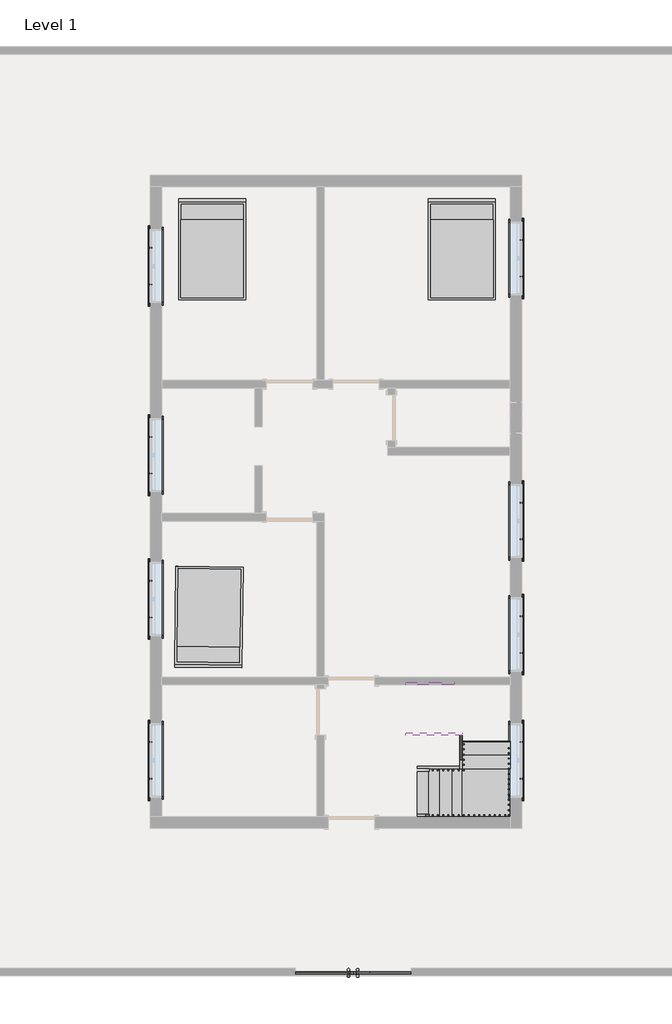
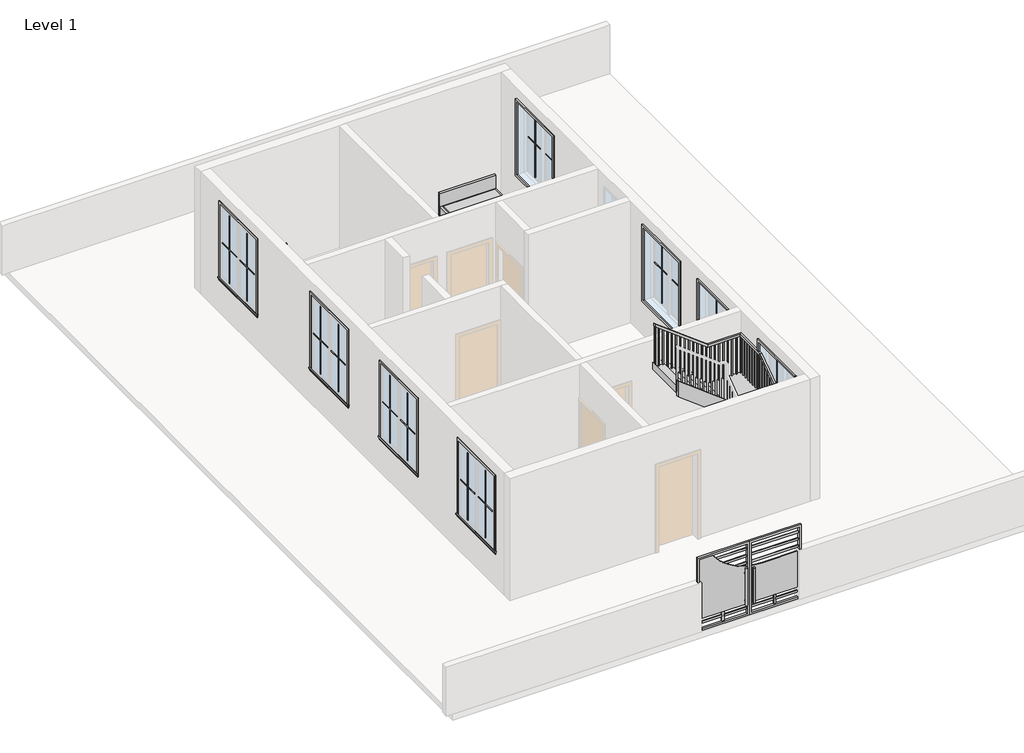
# One storey, part 2 of 2: 33 proxies, 5 members, 3 furniture elements, 1 railing, 1 stair flight.
"""IFC4 building model written with IfcOpenShell, lengths in millimetres."""

from ifc_helpers import new_model, si_unit, frame, origin, place, context, project, spatial, polyline, outline, extrude, faceted_brep, transform, mapped, element, save
from components import generic_models_113f6068, muntin_pattern_2x2_muntin_pattern_2x2_bff912c5, muntin_pattern_2x2_muntin_pattern_2x2_c2194282, trim_window_exterior_flat_with_sill_e04b3088, trim_window_interior_flat_picture_frame_2a7685fe, bed_17739_bed_17739_15c61121, stair_flight_3d22c4e0

model = new_model("IFC4")

# Units and contexts
model_context = context("Model", 3, world=origin())
ifc_project = project(units=[si_unit("LENGTHUNIT", "METRE", prefix="MILLI")], contexts=[model_context])

# Site, building, storey
site = spatial("IfcSite", under=ifc_project)
building = spatial("IfcBuilding", under=site)
storey = spatial("IfcBuildingStorey", under=building, Name="Level 1", Elevation=0.0)

# Proxies
placement = place(None, origin())
generic_models_shape = generic_models_113f6068(model_context)
element("IfcBuildingElementProxy", 1, Name="Generic Models", at=placement, inside=storey, context=model_context, shape_type="MappedRepresentation", body=[
    mapped(generic_models_shape, transform((-917.7018997, -9199.4071712, 0.0), x_axis=(1.0, 0.0, 0.0), y_axis=(0.0, 1.0, 0.0), z_axis=(0.0, 0.0, 1.0))),
])
muntin_pattern_2x2_muntin_pattern_2x2_shape = muntin_pattern_2x2_muntin_pattern_2x2_bff912c5(model_context)
element("IfcBuildingElementProxy", 2, Name="Muntin Pattern_2x2 : Muntin Pattern_2x2", ObjectType="Muntin Pattern_2x2 : Muntin Pattern_2x2", at=placement, inside=storey, context=model_context, shape_type="MappedRepresentation", body=[
    mapped(muntin_pattern_2x2_muntin_pattern_2x2_shape, transform((-4903.510885, -5396.5975571, 984.25), x_axis=(0.0, 1.0, 0.0), y_axis=(-1.0, 0.0, 0.0), z_axis=(0.0, 0.0, 1.0))),
])
element("IfcBuildingElementProxy", 3, Name="Muntin Pattern_2x2 : Muntin Pattern_2x2", ObjectType="Muntin Pattern_2x2 : Muntin Pattern_2x2", at=placement, inside=storey, context=model_context, shape_type="MappedRepresentation", body=[
    mapped(muntin_pattern_2x2_muntin_pattern_2x2_shape, transform((2392.639115, -4675.8725571, 984.25), x_axis=(0.0, -1.0, 0.0), y_axis=(1.0, 0.0, 0.0), z_axis=(0.0, 0.0, 1.0))),
])
element("IfcBuildingElementProxy", 4, Name="Muntin Pattern_2x2 : Muntin Pattern_2x2", ObjectType="Muntin Pattern_2x2 : Muntin Pattern_2x2", at=placement, inside=storey, context=model_context, shape_type="MappedRepresentation", body=[
    mapped(muntin_pattern_2x2_muntin_pattern_2x2_shape, transform((2392.639115, -2199.3725571, 984.25), x_axis=(0.0, -1.0, 0.0), y_axis=(1.0, 0.0, 0.0), z_axis=(0.0, 0.0, 1.0))),
])
element("IfcBuildingElementProxy", 5, Name="Muntin Pattern_2x2 : Muntin Pattern_2x2", ObjectType="Muntin Pattern_2x2 : Muntin Pattern_2x2", at=placement, inside=storey, context=model_context, shape_type="MappedRepresentation", body=[
    mapped(muntin_pattern_2x2_muntin_pattern_2x2_shape, transform((2392.639115, 35.8274429, 984.25), x_axis=(0.0, -1.0, 0.0), y_axis=(1.0, 0.0, 0.0), z_axis=(0.0, 0.0, 1.0))),
])
element("IfcBuildingElementProxy", 6, Name="Muntin Pattern_2x2 : Muntin Pattern_2x2", ObjectType="Muntin Pattern_2x2 : Muntin Pattern_2x2", at=placement, inside=storey, context=model_context, shape_type="MappedRepresentation", body=[
    mapped(muntin_pattern_2x2_muntin_pattern_2x2_shape, transform((-4903.510885, -2221.5975571, 984.25), x_axis=(0.0, 1.0, 0.0), y_axis=(-1.0, 0.0, 0.0), z_axis=(0.0, 0.0, 1.0))),
])
element("IfcBuildingElementProxy", 7, Name="Muntin Pattern_2x2 : Muntin Pattern_2x2", ObjectType="Muntin Pattern_2x2 : Muntin Pattern_2x2", at=placement, inside=storey, context=model_context, shape_type="MappedRepresentation", body=[
    mapped(muntin_pattern_2x2_muntin_pattern_2x2_shape, transform((-4903.510885, 610.5024429, 984.25), x_axis=(0.0, 1.0, 0.0), y_axis=(-1.0, 0.0, 0.0), z_axis=(0.0, 0.0, 1.0))),
])
element("IfcBuildingElementProxy", 8, Name="Muntin Pattern_2x2 : Muntin Pattern_2x2", ObjectType="Muntin Pattern_2x2 : Muntin Pattern_2x2", at=placement, inside=storey, context=model_context, shape_type="MappedRepresentation", body=[
    mapped(muntin_pattern_2x2_muntin_pattern_2x2_shape, transform((-4903.510885, 4331.6024429, 984.25), x_axis=(0.0, 1.0, 0.0), y_axis=(-1.0, 0.0, 0.0), z_axis=(0.0, 0.0, 1.0))),
])
element("IfcBuildingElementProxy", 9, Name="Muntin Pattern_2x2 : Muntin Pattern_2x2", ObjectType="Muntin Pattern_2x2 : Muntin Pattern_2x2", at=placement, inside=storey, context=model_context, shape_type="MappedRepresentation", body=[
    mapped(muntin_pattern_2x2_muntin_pattern_2x2_shape, transform((2392.639115, 5204.7274429, 984.25), x_axis=(0.0, -1.0, 0.0), y_axis=(1.0, 0.0, 0.0), z_axis=(0.0, 0.0, 1.0))),
])
muntin_pattern_2x2_muntin_pattern_2x2_2_shape = muntin_pattern_2x2_muntin_pattern_2x2_c2194282(model_context)
element("IfcBuildingElementProxy", 10, Name="Muntin Pattern_2x2 : Muntin Pattern_2x2", ObjectType="Muntin Pattern_2x2 : Muntin Pattern_2x2", at=placement, inside=storey, context=model_context, shape_type="MappedRepresentation", body=[
    mapped(muntin_pattern_2x2_muntin_pattern_2x2_2_shape, transform((-4903.510885, -4675.8725571, 984.25), x_axis=(0.0, -1.0, 0.0), y_axis=(1.0, 0.0, 0.0), z_axis=(0.0, 0.0, 1.0))),
])
element("IfcBuildingElementProxy", 11, Name="Muntin Pattern_2x2 : Muntin Pattern_2x2", ObjectType="Muntin Pattern_2x2 : Muntin Pattern_2x2", at=placement, inside=storey, context=model_context, shape_type="MappedRepresentation", body=[
    mapped(muntin_pattern_2x2_muntin_pattern_2x2_2_shape, transform((2392.639115, -5396.5975571, 984.25), x_axis=(0.0, 1.0, 0.0), y_axis=(-1.0, 0.0, 0.0), z_axis=(0.0, 0.0, 1.0))),
])
element("IfcBuildingElementProxy", 12, Name="Muntin Pattern_2x2 : Muntin Pattern_2x2", ObjectType="Muntin Pattern_2x2 : Muntin Pattern_2x2", at=placement, inside=storey, context=model_context, shape_type="MappedRepresentation", body=[
    mapped(muntin_pattern_2x2_muntin_pattern_2x2_2_shape, transform((2392.639115, -2920.0975571, 984.25), x_axis=(0.0, 1.0, 0.0), y_axis=(-1.0, 0.0, 0.0), z_axis=(0.0, 0.0, 1.0))),
])
element("IfcBuildingElementProxy", 13, Name="Muntin Pattern_2x2 : Muntin Pattern_2x2", ObjectType="Muntin Pattern_2x2 : Muntin Pattern_2x2", at=placement, inside=storey, context=model_context, shape_type="MappedRepresentation", body=[
    mapped(muntin_pattern_2x2_muntin_pattern_2x2_2_shape, transform((2392.639115, -684.8975571, 984.25), x_axis=(0.0, 1.0, 0.0), y_axis=(-1.0, 0.0, 0.0), z_axis=(0.0, 0.0, 1.0))),
])
element("IfcBuildingElementProxy", 14, Name="Muntin Pattern_2x2 : Muntin Pattern_2x2", ObjectType="Muntin Pattern_2x2 : Muntin Pattern_2x2", at=placement, inside=storey, context=model_context, shape_type="MappedRepresentation", body=[
    mapped(muntin_pattern_2x2_muntin_pattern_2x2_2_shape, transform((-4903.510885, -1500.8725571, 984.25), x_axis=(0.0, -1.0, 0.0), y_axis=(1.0, 0.0, 0.0), z_axis=(0.0, 0.0, 1.0))),
])
element("IfcBuildingElementProxy", 15, Name="Muntin Pattern_2x2 : Muntin Pattern_2x2", ObjectType="Muntin Pattern_2x2 : Muntin Pattern_2x2", at=placement, inside=storey, context=model_context, shape_type="MappedRepresentation", body=[
    mapped(muntin_pattern_2x2_muntin_pattern_2x2_2_shape, transform((-4903.510885, 1331.2274429, 984.25), x_axis=(0.0, -1.0, 0.0), y_axis=(1.0, 0.0, 0.0), z_axis=(0.0, 0.0, 1.0))),
])
element("IfcBuildingElementProxy", 16, Name="Muntin Pattern_2x2 : Muntin Pattern_2x2", ObjectType="Muntin Pattern_2x2 : Muntin Pattern_2x2", at=placement, inside=storey, context=model_context, shape_type="MappedRepresentation", body=[
    mapped(muntin_pattern_2x2_muntin_pattern_2x2_2_shape, transform((-4903.510885, 5052.3274429, 984.25), x_axis=(0.0, -1.0, 0.0), y_axis=(1.0, 0.0, 0.0), z_axis=(0.0, 0.0, 1.0))),
])
element("IfcBuildingElementProxy", 17, Name="Muntin Pattern_2x2 : Muntin Pattern_2x2", ObjectType="Muntin Pattern_2x2 : Muntin Pattern_2x2", at=placement, inside=storey, context=model_context, shape_type="MappedRepresentation", body=[
    mapped(muntin_pattern_2x2_muntin_pattern_2x2_2_shape, transform((2392.639115, 4484.0024429, 984.25), x_axis=(0.0, 1.0, 0.0), y_axis=(-1.0, 0.0, 0.0), z_axis=(0.0, 0.0, 1.0))),
])
trim_window_exterior_flat_with_sill_shape = trim_window_exterior_flat_with_sill_e04b3088(model_context)
element("IfcBuildingElementProxy", 18, Name="Trim-Window-Exterior-Flat : with Sill", ObjectType="Trim-Window-Exterior-Flat : with Sill", at=placement, inside=storey, context=model_context, shape_type="MappedRepresentation", body=[
    mapped(trim_window_exterior_flat_with_sill_shape, transform((-4913.035885, -5036.2350571, 2743.2), x_axis=(0.0, -1.0, 0.0), y_axis=(0.0, 0.0, 1.0), z_axis=(-1.0, 0.0, 0.0))),
])
element("IfcBuildingElementProxy", 19, Name="Trim-Window-Exterior-Flat : with Sill", ObjectType="Trim-Window-Exterior-Flat : with Sill", at=placement, inside=storey, context=model_context, shape_type="MappedRepresentation", body=[
    mapped(trim_window_exterior_flat_with_sill_shape, transform((2402.164115, -5036.2350571, 2743.2), x_axis=(0.0, 1.0, 0.0), y_axis=(0.0, 0.0, 1.0), z_axis=(1.0, 0.0, 0.0))),
])
element("IfcBuildingElementProxy", 20, Name="Trim-Window-Exterior-Flat : with Sill", ObjectType="Trim-Window-Exterior-Flat : with Sill", at=placement, inside=storey, context=model_context, shape_type="MappedRepresentation", body=[
    mapped(trim_window_exterior_flat_with_sill_shape, transform((2402.164115, -2559.7350571, 2743.2), x_axis=(0.0, 1.0, 0.0), y_axis=(0.0, 0.0, 1.0), z_axis=(1.0, 0.0, 0.0))),
])
element("IfcBuildingElementProxy", 21, Name="Trim-Window-Exterior-Flat : with Sill", ObjectType="Trim-Window-Exterior-Flat : with Sill", at=placement, inside=storey, context=model_context, shape_type="MappedRepresentation", body=[
    mapped(trim_window_exterior_flat_with_sill_shape, transform((2402.164115, -324.5350571, 2743.2), x_axis=(0.0, 1.0, 0.0), y_axis=(0.0, 0.0, 1.0), z_axis=(1.0, 0.0, 0.0))),
])
element("IfcBuildingElementProxy", 22, Name="Trim-Window-Exterior-Flat : with Sill", ObjectType="Trim-Window-Exterior-Flat : with Sill", at=placement, inside=storey, context=model_context, shape_type="MappedRepresentation", body=[
    mapped(trim_window_exterior_flat_with_sill_shape, transform((-4913.035885, -1861.2350571, 2743.2), x_axis=(0.0, -1.0, 0.0), y_axis=(0.0, 0.0, 1.0), z_axis=(-1.0, 0.0, 0.0))),
])
element("IfcBuildingElementProxy", 23, Name="Trim-Window-Exterior-Flat : with Sill", ObjectType="Trim-Window-Exterior-Flat : with Sill", at=placement, inside=storey, context=model_context, shape_type="MappedRepresentation", body=[
    mapped(trim_window_exterior_flat_with_sill_shape, transform((-4913.035885, 970.8649429, 2743.2), x_axis=(0.0, -1.0, 0.0), y_axis=(0.0, 0.0, 1.0), z_axis=(-1.0, 0.0, 0.0))),
])
element("IfcBuildingElementProxy", 24, Name="Trim-Window-Exterior-Flat : with Sill", ObjectType="Trim-Window-Exterior-Flat : with Sill", at=placement, inside=storey, context=model_context, shape_type="MappedRepresentation", body=[
    mapped(trim_window_exterior_flat_with_sill_shape, transform((-4913.035885, 4691.9649429, 2743.2), x_axis=(0.0, -1.0, 0.0), y_axis=(0.0, 0.0, 1.0), z_axis=(-1.0, 0.0, 0.0))),
])
element("IfcBuildingElementProxy", 25, Name="Trim-Window-Exterior-Flat : with Sill", ObjectType="Trim-Window-Exterior-Flat : with Sill", at=placement, inside=storey, context=model_context, shape_type="MappedRepresentation", body=[
    mapped(trim_window_exterior_flat_with_sill_shape, transform((2402.164115, 4844.3649429, 2743.2), x_axis=(0.0, 1.0, 0.0), y_axis=(0.0, 0.0, 1.0), z_axis=(1.0, 0.0, 0.0))),
])
trim_window_interior_flat_picture_frame_shape = trim_window_interior_flat_picture_frame_2a7685fe(model_context)
element("IfcBuildingElementProxy", 26, Name="Trim-Window-Interior-Flat : Picture Frame", ObjectType="Trim-Window-Interior-Flat : Picture Frame", at=placement, inside=storey, context=model_context, shape_type="MappedRepresentation", body=[
    mapped(trim_window_interior_flat_picture_frame_shape, transform((-4684.435885, -5036.2350571, 2743.2), x_axis=(0.0, 1.0, 0.0), y_axis=(0.0, 0.0, 1.0), z_axis=(1.0, 0.0, 0.0))),
])
element("IfcBuildingElementProxy", 27, Name="Trim-Window-Interior-Flat : Picture Frame", ObjectType="Trim-Window-Interior-Flat : Picture Frame", at=placement, inside=storey, context=model_context, shape_type="MappedRepresentation", body=[
    mapped(trim_window_interior_flat_picture_frame_shape, transform((2173.564115, -5036.2350571, 2743.2), x_axis=(0.0, -1.0, 0.0), y_axis=(0.0, 0.0, 1.0), z_axis=(-1.0, 0.0, 0.0))),
])
element("IfcBuildingElementProxy", 28, Name="Trim-Window-Interior-Flat : Picture Frame", ObjectType="Trim-Window-Interior-Flat : Picture Frame", at=placement, inside=storey, context=model_context, shape_type="MappedRepresentation", body=[
    mapped(trim_window_interior_flat_picture_frame_shape, transform((2173.564115, -2559.7350571, 2743.2), x_axis=(0.0, -1.0, 0.0), y_axis=(0.0, 0.0, 1.0), z_axis=(-1.0, 0.0, 0.0))),
])
element("IfcBuildingElementProxy", 29, Name="Trim-Window-Interior-Flat : Picture Frame", ObjectType="Trim-Window-Interior-Flat : Picture Frame", at=placement, inside=storey, context=model_context, shape_type="MappedRepresentation", body=[
    mapped(trim_window_interior_flat_picture_frame_shape, transform((2173.564115, -324.5350571, 2743.2), x_axis=(0.0, -1.0, 0.0), y_axis=(0.0, 0.0, 1.0), z_axis=(-1.0, 0.0, 0.0))),
])
element("IfcBuildingElementProxy", 30, Name="Trim-Window-Interior-Flat : Picture Frame", ObjectType="Trim-Window-Interior-Flat : Picture Frame", at=placement, inside=storey, context=model_context, shape_type="MappedRepresentation", body=[
    mapped(trim_window_interior_flat_picture_frame_shape, transform((-4684.435885, -1861.2350571, 2743.2), x_axis=(0.0, 1.0, 0.0), y_axis=(0.0, 0.0, 1.0), z_axis=(1.0, 0.0, 0.0))),
])
element("IfcBuildingElementProxy", 31, Name="Trim-Window-Interior-Flat : Picture Frame", ObjectType="Trim-Window-Interior-Flat : Picture Frame", at=placement, inside=storey, context=model_context, shape_type="MappedRepresentation", body=[
    mapped(trim_window_interior_flat_picture_frame_shape, transform((-4684.435885, 970.8649429, 2743.2), x_axis=(0.0, 1.0, 0.0), y_axis=(0.0, 0.0, 1.0), z_axis=(1.0, 0.0, 0.0))),
])
element("IfcBuildingElementProxy", 32, Name="Trim-Window-Interior-Flat : Picture Frame", ObjectType="Trim-Window-Interior-Flat : Picture Frame", at=placement, inside=storey, context=model_context, shape_type="MappedRepresentation", body=[
    mapped(trim_window_interior_flat_picture_frame_shape, transform((-4684.435885, 4691.9649429, 2743.2), x_axis=(0.0, 1.0, 0.0), y_axis=(0.0, 0.0, 1.0), z_axis=(1.0, 0.0, 0.0))),
])
element("IfcBuildingElementProxy", 33, Name="Trim-Window-Interior-Flat : Picture Frame", ObjectType="Trim-Window-Interior-Flat : Picture Frame", at=placement, inside=storey, context=model_context, shape_type="MappedRepresentation", body=[
    mapped(trim_window_interior_flat_picture_frame_shape, transform((2173.564115, 4844.3649429, 2743.2), x_axis=(0.0, -1.0, 0.0), y_axis=(0.0, 0.0, 1.0), z_axis=(-1.0, 0.0, 0.0))),
])

# Furniture
bed_17739_bed_17739_shape = bed_17739_bed_17739_15c61121(model_context)
element("IfcFurniture", 34, ObjectType="Bed_17739 : Bed_17739", at=placement, inside=storey, context=model_context, shape_type="MappedRepresentation", body=[
    mapped(bed_17739_bed_17739_shape, transform((-3693.835885, 4996.7649429, 0.0), x_axis=(1.0, 0.0, 0.0), y_axis=(0.0, 1.0, 0.0), z_axis=(0.0, 0.0, 1.0))),
])
element("IfcFurniture", 35, ObjectType="Bed_17739 : Bed_17739", at=placement, inside=storey, context=model_context, shape_type="MappedRepresentation", body=[
    mapped(bed_17739_bed_17739_shape, transform((1221.064115, 4996.7649429, 0.0), x_axis=(1.0, 0.0, 0.0), y_axis=(0.0, 1.0, 0.0), z_axis=(0.0, 0.0, 1.0))),
])
element("IfcFurniture", 36, ObjectType="Bed_17739 : Bed_17739", at=placement, inside=storey, context=model_context, shape_type="MappedRepresentation", body=[
    mapped(bed_17739_bed_17739_shape, transform((-3756.0321663, -2189.364606, 0.0), x_axis=(-0.9999334593473937, 0.011535895177843815, 0.0), y_axis=(-0.011535895177843815, -0.9999334593473937, 0.0), z_axis=(0.0, 0.0, 1.0))),
])

# Members
element("IfcMember", 37, ObjectType="Stringer - 2\" Width", at=placement, inside=storey, context=model_context, shape_type="SweptSolid", body=[
    extrude(outline(polyline([(222.6959685, 344.764115), (0.0, 344.764115), (0.0, 555.1685253), (482.9196844, 1182.964115), (867.4651993, 1182.964115), (222.6959685, 344.764115)])), frame((0.0, -5201.3350571, 0.0), z_axis=(0.0, 1.0, 0.0), x_axis=(0.0, 0.0, 1.0)), (0.0, 0.0, 1.0), 50.8),
])
element("IfcMember", 38, ObjectType="Stringer - 2\" Width", at=placement, inside=storey, context=model_context, shape_type="SweptSolid", body=[
    extrude(outline(polyline([(-5201.3350571, 695.152716), (-5201.3350571, 1069.7225362), (-4540.9350571, 1541.4368219), (-4540.9350571, 1166.8670017), (-5201.3350571, 695.152716)])), frame((1182.964115, 0.0, 0.0), z_axis=(1.0, 0.0, 0.0), x_axis=(0.0, 1.0, 0.0)), (0.0, 0.0, 1.0), 50.8),
])
element("IfcMember", 39, ObjectType="Stringer - 2\" Width", at=placement, inside=storey, context=model_context, shape_type="SweptSolid", body=[
    extrude(outline(polyline([(1369.1786616, 1233.764115), (1752.3668, 1233.764115), (2603.8715619, 116.164115), (2220.6834236, 116.164115), (1369.1786616, 1233.764115)])), frame((0.0, -4540.9350571, 0.0), z_axis=(0.0, 1.0, 0.0), x_axis=(0.0, 0.0, 1.0)), (0.0, 0.0, 1.0), 50.8),
])
element("IfcMember", 40, ObjectType="Stringer - 2\" Width", at=placement, inside=storey, context=model_context, shape_type="SweptSolid", body=[
    extrude(outline(polyline([(222.6959685, 344.764115), (0.0, 344.764115), (0.0, 555.1685253), (398.4368219, 1073.1363938), (398.4368219, 573.2272245), (222.6959685, 344.764115)])), frame((0.0, -6191.9350571, 0.0), z_axis=(0.0, 1.0, 0.0), x_axis=(0.0, 0.0, 1.0)), (0.0, 0.0, 1.0), 50.8),
])
element("IfcMember", 41, ObjectType="Stringer - 2\" Width", at=placement, inside=storey, context=model_context, shape_type="SweptSolid", body=[
    extrude(outline(polyline([(1874.4384303, 1073.5451003), (2603.8715619, 116.164115), (2220.6834236, 116.164115), (1874.4384303, 570.6106687), (1874.4384303, 1073.5451003)])), frame((0.0, -3550.3350571, 0.0), z_axis=(0.0, 1.0, 0.0), x_axis=(0.0, 0.0, 1.0)), (0.0, 0.0, 1.0), 50.8),
])

# Railing
element("IfcRailing", 42, ObjectType="Handrail - Rectangular", at=placement, inside=storey, context=model_context, shape_type="SolidModel", body=[
    faceted_brep([(344.764115, -6090.3350571, 1083.7333333), (344.764115, -6090.3350571, 1019.8686436), (344.764115, -6141.1350571, 1019.8686436), (344.764115, -6141.1350571, 1083.7333333), (1373.464115, -6090.3350571, 1867.5047619), (1390.6115203, -6090.3350571, 1816.7047619), (1390.6115203, -6141.1350571, 1816.7047619), (1373.464115, -6141.1350571, 1867.5047619), (2122.764115, -6090.3350571, 1867.5047619), (2122.764115, -6090.3350571, 1816.7047619), (2173.564115, -6141.1350571, 1816.7047619), (2173.564115, -6141.1350571, 1867.5047619), (2122.764115, -5289.3883904, 1867.5047619), (2122.764115, -5273.1087657, 1816.7047619), (2173.564115, -5273.1087657, 1816.7047619), (2173.564115, -5289.3883904, 1867.5047619), (2122.764115, -4399.3108146, 2503.2744589), (2122.764115, -4383.0311899, 2452.4744589), (2173.564115, -4383.0311899, 2452.4744589), (2173.564115, -4399.3108146, 2503.2744589), (2122.764115, -3601.1350571, 2503.2744589), (2122.764115, -3601.1350571, 2452.4744589), (2173.564115, -3550.3350571, 2452.4744589), (2173.564115, -3550.3350571, 2503.2744589), (1371.6498293, -3601.1350571, 2503.2744589), (1354.5800477, -3601.1350571, 2452.4744589), (1354.5800477, -3550.3350571, 2452.4744589), (1371.6498293, -3550.3350571, 2503.2744589), (116.164115, -3601.1350571, 3454.4), (116.164115, -3550.3350571, 3454.4), (116.164115, -3550.3350571, 3390.6683472), (116.164115, -3601.1350571, 3390.6683472)], [[[0, 1, 2, 3]], [[1, 0, 4, 5]], [[2, 1, 5, 6]], [[3, 2, 6, 7]], [[0, 3, 7, 4]], [[5, 4, 8, 9]], [[6, 5, 9, 10]], [[7, 6, 10, 11]], [[4, 7, 11, 8]], [[9, 8, 12, 13]], [[10, 9, 13, 14]], [[11, 10, 14, 15]], [[8, 11, 15, 12]], [[13, 12, 16, 17]], [[14, 13, 17, 18]], [[15, 14, 18, 19]], [[12, 15, 19, 16]], [[17, 16, 20, 21]], [[18, 17, 21, 22]], [[19, 18, 22, 23]], [[16, 19, 23, 20]], [[21, 20, 24, 25]], [[22, 21, 25, 26]], [[23, 22, 26, 27]], [[20, 23, 27, 24]], [[28, 29, 30, 31]], [[25, 24, 28, 31]], [[26, 25, 31, 30]], [[27, 26, 30, 29]], [[24, 27, 29, 28]]]),
    extrude(outline(polyline([(3306.4827412, 227.289115), (3320.9145594, 208.239115), (2370.6666667, 208.239115), (2370.6666667, 227.289115), (3306.4827412, 227.289115)])), frame((0.0, -3585.2600571, 0.0), z_axis=(0.0, 1.0, 0.0), x_axis=(0.0, 0.0, 1.0)), (0.0, 0.0, 1.0), 19.05),
    extrude(outline(polyline([(3229.5130442, 328.889115), (3243.9448624, 309.839115), (2370.6666667, 309.839115), (2370.6666667, 328.889115), (3229.5130442, 328.889115)])), frame((0.0, -3585.2600571, 0.0), z_axis=(0.0, 1.0, 0.0), x_axis=(0.0, 0.0, 1.0)), (0.0, 0.0, 1.0), 19.05),
    extrude(outline(polyline([(3152.5433472, 430.489115), (3166.9751654, 411.439115), (2201.3333333, 411.439115), (2201.3333333, 430.489115), (3152.5433472, 430.489115)])), frame((0.0, -3585.2600571, 0.0), z_axis=(0.0, 1.0, 0.0), x_axis=(0.0, 0.0, 1.0)), (0.0, 0.0, 1.0), 19.05),
    extrude(outline(polyline([(3075.5736503, 532.089115), (3090.0054685, 513.039115), (2201.3333333, 513.039115), (2201.3333333, 532.089115), (3075.5736503, 532.089115)])), frame((0.0, -3585.2600571, 0.0), z_axis=(0.0, 1.0, 0.0), x_axis=(0.0, 0.0, 1.0)), (0.0, 0.0, 1.0), 19.05),
    extrude(outline(polyline([(2998.6039533, 633.689115), (3013.0357715, 614.639115), (2032.0, 614.639115), (2032.0, 633.689115), (2998.6039533, 633.689115)])), frame((0.0, -3585.2600571, 0.0), z_axis=(0.0, 1.0, 0.0), x_axis=(0.0, 0.0, 1.0)), (0.0, 0.0, 1.0), 19.05),
    extrude(outline(polyline([(2921.6342563, 735.289115), (2936.0660745, 716.239115), (2032.0, 716.239115), (2032.0, 735.289115), (2921.6342563, 735.289115)])), frame((0.0, -3585.2600571, 0.0), z_axis=(0.0, 1.0, 0.0), x_axis=(0.0, 0.0, 1.0)), (0.0, 0.0, 1.0), 19.05),
    extrude(outline(polyline([(2844.6645594, 836.889115), (2859.0963775, 817.839115), (1862.6666667, 817.839115), (1862.6666667, 836.889115), (2844.6645594, 836.889115)])), frame((0.0, -3585.2600571, 0.0), z_axis=(0.0, 1.0, 0.0), x_axis=(0.0, 0.0, 1.0)), (0.0, 0.0, 1.0), 19.05),
    extrude(outline(polyline([(2767.6948624, 938.489115), (2782.1266806, 919.439115), (1862.6666667, 919.439115), (1862.6666667, 938.489115), (2767.6948624, 938.489115)])), frame((0.0, -3585.2600571, 0.0), z_axis=(0.0, 1.0, 0.0), x_axis=(0.0, 0.0, 1.0)), (0.0, 0.0, 1.0), 19.05),
    extrude(outline(polyline([(2690.7251654, 1040.089115), (2705.1569836, 1021.039115), (1862.6666667, 1021.039115), (1862.6666667, 1040.089115), (2690.7251654, 1040.089115)])), frame((0.0, -3585.2600571, 0.0), z_axis=(0.0, 1.0, 0.0), x_axis=(0.0, 0.0, 1.0)), (0.0, 0.0, 1.0), 19.05),
    extrude(outline(polyline([(2613.7554685, 1141.689115), (2628.1872866, 1122.639115), (1693.3333333, 1122.639115), (1693.3333333, 1141.689115), (2613.7554685, 1141.689115)])), frame((0.0, -3585.2600571, 0.0), z_axis=(0.0, 1.0, 0.0), x_axis=(0.0, 0.0, 1.0)), (0.0, 0.0, 1.0), 19.05),
    extrude(outline(polyline([(2536.7857715, 1243.289115), (2551.2175897, 1224.239115), (1693.3333333, 1224.239115), (1693.3333333, 1243.289115), (2536.7857715, 1243.289115)])), frame((0.0, -3585.2600571, 0.0), z_axis=(0.0, 1.0, 0.0), x_axis=(0.0, 0.0, 1.0)), (0.0, 0.0, 1.0), 19.05),
    extrude(outline(polyline([(2459.8160745, 1344.889115), (2474.2478927, 1325.839115), (1524.0, 1325.839115), (1524.0, 1344.889115), (2459.8160745, 1344.889115)])), frame((0.0, -3585.2600571, 0.0), z_axis=(0.0, 1.0, 0.0), x_axis=(0.0, 0.0, 1.0)), (0.0, 0.0, 1.0), 19.05),
    extrude(outline(polyline([(1446.489115, -3566.2100571), (1446.489115, -3585.2600571), (1427.439115, -3585.2600571), (1427.439115, -3566.2100571), (1446.489115, -3566.2100571)])), frame((0.0, 0.0, 1524.0), z_axis=(0.0, 0.0, 1.0), x_axis=(1.0, 0.0, 0.0)), (0.0, 0.0, 1.0), 928.4744589),
    extrude(outline(polyline([(1548.089115, -3566.2100571), (1548.089115, -3585.2600571), (1529.039115, -3585.2600571), (1529.039115, -3566.2100571), (1548.089115, -3566.2100571)])), frame((0.0, 0.0, 1524.0), z_axis=(0.0, 0.0, 1.0), x_axis=(1.0, 0.0, 0.0)), (0.0, 0.0, 1.0), 928.4744589),
    extrude(outline(polyline([(1649.689115, -3566.2100571), (1649.689115, -3585.2600571), (1630.639115, -3585.2600571), (1630.639115, -3566.2100571), (1649.689115, -3566.2100571)])), frame((0.0, 0.0, 1524.0), z_axis=(0.0, 0.0, 1.0), x_axis=(1.0, 0.0, 0.0)), (0.0, 0.0, 1.0), 928.4744589),
    extrude(outline(polyline([(1751.289115, -3566.2100571), (1751.289115, -3585.2600571), (1732.239115, -3585.2600571), (1732.239115, -3566.2100571), (1751.289115, -3566.2100571)])), frame((0.0, 0.0, 1524.0), z_axis=(0.0, 0.0, 1.0), x_axis=(1.0, 0.0, 0.0)), (0.0, 0.0, 1.0), 928.4744589),
    extrude(outline(polyline([(1852.889115, -3566.2100571), (1852.889115, -3585.2600571), (1833.839115, -3585.2600571), (1833.839115, -3566.2100571), (1852.889115, -3566.2100571)])), frame((0.0, 0.0, 1524.0), z_axis=(0.0, 0.0, 1.0), x_axis=(1.0, 0.0, 0.0)), (0.0, 0.0, 1.0), 928.4744589),
    extrude(outline(polyline([(1954.489115, -3566.2100571), (1954.489115, -3585.2600571), (1935.439115, -3585.2600571), (1935.439115, -3566.2100571), (1954.489115, -3566.2100571)])), frame((0.0, 0.0, 1524.0), z_axis=(0.0, 0.0, 1.0), x_axis=(1.0, 0.0, 0.0)), (0.0, 0.0, 1.0), 928.4744589),
    extrude(outline(polyline([(2056.089115, -3566.2100571), (2056.089115, -3585.2600571), (2037.039115, -3585.2600571), (2037.039115, -3566.2100571), (2056.089115, -3566.2100571)])), frame((0.0, 0.0, 1524.0), z_axis=(0.0, 0.0, 1.0), x_axis=(1.0, 0.0, 0.0)), (0.0, 0.0, 1.0), 928.4744589),
    extrude(outline(polyline([(2157.689115, -3686.8600571), (2138.639115, -3686.8600571), (2138.639115, -3667.8100571), (2157.689115, -3667.8100571), (2157.689115, -3686.8600571)])), frame((0.0, 0.0, 1524.0), z_axis=(0.0, 0.0, 1.0), x_axis=(1.0, 0.0, 0.0)), (0.0, 0.0, 1.0), 928.4744589),
    extrude(outline(polyline([(2157.689115, -3788.4600571), (2138.639115, -3788.4600571), (2138.639115, -3769.4100571), (2157.689115, -3769.4100571), (2157.689115, -3788.4600571)])), frame((0.0, 0.0, 1524.0), z_axis=(0.0, 0.0, 1.0), x_axis=(1.0, 0.0, 0.0)), (0.0, 0.0, 1.0), 928.4744589),
    extrude(outline(polyline([(2157.689115, -3890.0600571), (2138.639115, -3890.0600571), (2138.639115, -3871.0100571), (2157.689115, -3871.0100571), (2157.689115, -3890.0600571)])), frame((0.0, 0.0, 1524.0), z_axis=(0.0, 0.0, 1.0), x_axis=(1.0, 0.0, 0.0)), (0.0, 0.0, 1.0), 928.4744589),
    extrude(outline(polyline([(2157.689115, -3991.6600571), (2138.639115, -3991.6600571), (2138.639115, -3972.6100571), (2157.689115, -3972.6100571), (2157.689115, -3991.6600571)])), frame((0.0, 0.0, 1524.0), z_axis=(0.0, 0.0, 1.0), x_axis=(1.0, 0.0, 0.0)), (0.0, 0.0, 1.0), 928.4744589),
    extrude(outline(polyline([(2157.689115, -4093.2600571), (2138.639115, -4093.2600571), (2138.639115, -4074.2100571), (2157.689115, -4074.2100571), (2157.689115, -4093.2600571)])), frame((0.0, 0.0, 1524.0), z_axis=(0.0, 0.0, 1.0), x_axis=(1.0, 0.0, 0.0)), (0.0, 0.0, 1.0), 928.4744589),
    extrude(outline(polyline([(2157.689115, -4194.8600571), (2138.639115, -4194.8600571), (2138.639115, -4175.8100571), (2157.689115, -4175.8100571), (2157.689115, -4194.8600571)])), frame((0.0, 0.0, 1524.0), z_axis=(0.0, 0.0, 1.0), x_axis=(1.0, 0.0, 0.0)), (0.0, 0.0, 1.0), 928.4744589),
    extrude(outline(polyline([(2157.689115, -4296.4600571), (2138.639115, -4296.4600571), (2138.639115, -4277.4100571), (2157.689115, -4277.4100571), (2157.689115, -4296.4600571)])), frame((0.0, 0.0, 1524.0), z_axis=(0.0, 0.0, 1.0), x_axis=(1.0, 0.0, 0.0)), (0.0, 0.0, 1.0), 928.4744589),
    extrude(outline(polyline([(2157.689115, -4398.0600571), (2138.639115, -4398.0600571), (2138.639115, -4379.0100571), (2157.689115, -4379.0100571), (2157.689115, -4398.0600571)])), frame((0.0, 0.0, 1524.0), z_axis=(0.0, 0.0, 1.0), x_axis=(1.0, 0.0, 0.0)), (0.0, 0.0, 1.0), 928.4744589),
    extrude(outline(polyline([(-4499.6600571, 2369.1681252), (-4480.6100571, 2382.7752681), (-4480.6100571, 1524.0), (-4499.6600571, 1524.0), (-4499.6600571, 2369.1681252)])), frame((2138.639115, 0.0, 0.0), z_axis=(1.0, 0.0, 0.0), x_axis=(0.0, 1.0, 0.0)), (0.0, 0.0, 1.0), 19.05),
    extrude(outline(polyline([(-4601.2600571, 2296.5966966), (-4582.2100571, 2310.2038395), (-4582.2100571, 1354.6666667), (-4601.2600571, 1354.6666667), (-4601.2600571, 2296.5966966)])), frame((2138.639115, 0.0, 0.0), z_axis=(1.0, 0.0, 0.0), x_axis=(0.0, 1.0, 0.0)), (0.0, 0.0, 1.0), 19.05),
    extrude(outline(polyline([(-4702.8600571, 2224.0252681), (-4683.8100571, 2237.6324109), (-4683.8100571, 1354.6666667), (-4702.8600571, 1354.6666667), (-4702.8600571, 2224.0252681)])), frame((2138.639115, 0.0, 0.0), z_axis=(1.0, 0.0, 0.0), x_axis=(0.0, 1.0, 0.0)), (0.0, 0.0, 1.0), 19.05),
    extrude(outline(polyline([(-4804.4600571, 2151.4538395), (-4785.4100571, 2165.0609823), (-4785.4100571, 1185.3333333), (-4804.4600571, 1185.3333333), (-4804.4600571, 2151.4538395)])), frame((2138.639115, 0.0, 0.0), z_axis=(1.0, 0.0, 0.0), x_axis=(0.0, 1.0, 0.0)), (0.0, 0.0, 1.0), 19.05),
    extrude(outline(polyline([(-4906.0600571, 2078.8824109), (-4887.0100571, 2092.4895538), (-4887.0100571, 1185.3333333), (-4906.0600571, 1185.3333333), (-4906.0600571, 2078.8824109)])), frame((2138.639115, 0.0, 0.0), z_axis=(1.0, 0.0, 0.0), x_axis=(0.0, 1.0, 0.0)), (0.0, 0.0, 1.0), 19.05),
    extrude(outline(polyline([(-5007.6600571, 2006.3109823), (-4988.6100571, 2019.9181252), (-4988.6100571, 1016.0), (-5007.6600571, 1016.0), (-5007.6600571, 2006.3109823)])), frame((2138.639115, 0.0, 0.0), z_axis=(1.0, 0.0, 0.0), x_axis=(0.0, 1.0, 0.0)), (0.0, 0.0, 1.0), 19.05),
    extrude(outline(polyline([(-5109.2600571, 1933.7395538), (-5090.2100571, 1947.3466966), (-5090.2100571, 1016.0), (-5109.2600571, 1016.0), (-5109.2600571, 1933.7395538)])), frame((2138.639115, 0.0, 0.0), z_axis=(1.0, 0.0, 0.0), x_axis=(0.0, 1.0, 0.0)), (0.0, 0.0, 1.0), 19.05),
    extrude(outline(polyline([(-5210.8600571, 1861.1681252), (-5191.8100571, 1874.7752681), (-5191.8100571, 1016.0), (-5210.8600571, 1016.0), (-5210.8600571, 1861.1681252)])), frame((2138.639115, 0.0, 0.0), z_axis=(1.0, 0.0, 0.0), x_axis=(0.0, 1.0, 0.0)), (0.0, 0.0, 1.0), 19.05),
    extrude(outline(polyline([(2157.689115, -5312.4600571), (2138.639115, -5312.4600571), (2138.639115, -5293.4100571), (2157.689115, -5293.4100571), (2157.689115, -5312.4600571)])), frame((0.0, 0.0, 846.6666667), z_axis=(0.0, 0.0, 1.0), x_axis=(1.0, 0.0, 0.0)), (0.0, 0.0, 1.0), 970.0380952),
    extrude(outline(polyline([(2157.689115, -5414.0600571), (2138.639115, -5414.0600571), (2138.639115, -5395.0100571), (2157.689115, -5395.0100571), (2157.689115, -5414.0600571)])), frame((0.0, 0.0, 846.6666667), z_axis=(0.0, 0.0, 1.0), x_axis=(1.0, 0.0, 0.0)), (0.0, 0.0, 1.0), 970.0380952),
    extrude(outline(polyline([(2157.689115, -5515.6600571), (2138.639115, -5515.6600571), (2138.639115, -5496.6100571), (2157.689115, -5496.6100571), (2157.689115, -5515.6600571)])), frame((0.0, 0.0, 846.6666667), z_axis=(0.0, 0.0, 1.0), x_axis=(1.0, 0.0, 0.0)), (0.0, 0.0, 1.0), 970.0380952),
    extrude(outline(polyline([(2157.689115, -5617.2600571), (2138.639115, -5617.2600571), (2138.639115, -5598.2100571), (2157.689115, -5598.2100571), (2157.689115, -5617.2600571)])), frame((0.0, 0.0, 846.6666667), z_axis=(0.0, 0.0, 1.0), x_axis=(1.0, 0.0, 0.0)), (0.0, 0.0, 1.0), 970.0380952),
    extrude(outline(polyline([(2157.689115, -5718.8600571), (2138.639115, -5718.8600571), (2138.639115, -5699.8100571), (2157.689115, -5699.8100571), (2157.689115, -5718.8600571)])), frame((0.0, 0.0, 846.6666667), z_axis=(0.0, 0.0, 1.0), x_axis=(1.0, 0.0, 0.0)), (0.0, 0.0, 1.0), 970.0380952),
    extrude(outline(polyline([(2157.689115, -5820.4600571), (2138.639115, -5820.4600571), (2138.639115, -5801.4100571), (2157.689115, -5801.4100571), (2157.689115, -5820.4600571)])), frame((0.0, 0.0, 846.6666667), z_axis=(0.0, 0.0, 1.0), x_axis=(1.0, 0.0, 0.0)), (0.0, 0.0, 1.0), 970.0380952),
    extrude(outline(polyline([(2157.689115, -5922.0600571), (2138.639115, -5922.0600571), (2138.639115, -5903.0100571), (2157.689115, -5903.0100571), (2157.689115, -5922.0600571)])), frame((0.0, 0.0, 846.6666667), z_axis=(0.0, 0.0, 1.0), x_axis=(1.0, 0.0, 0.0)), (0.0, 0.0, 1.0), 970.0380952),
    extrude(outline(polyline([(2157.689115, -6023.6600571), (2138.639115, -6023.6600571), (2138.639115, -6004.6100571), (2157.689115, -6004.6100571), (2157.689115, -6023.6600571)])), frame((0.0, 0.0, 846.6666667), z_axis=(0.0, 0.0, 1.0), x_axis=(1.0, 0.0, 0.0)), (0.0, 0.0, 1.0), 970.0380952),
    extrude(outline(polyline([(2062.439115, -6125.2600571), (2062.439115, -6106.2100571), (2081.489115, -6106.2100571), (2081.489115, -6125.2600571), (2062.439115, -6125.2600571)])), frame((0.0, 0.0, 846.6666667), z_axis=(0.0, 0.0, 1.0), x_axis=(1.0, 0.0, 0.0)), (0.0, 0.0, 1.0), 970.0380952),
    extrude(outline(polyline([(1960.839115, -6125.2600571), (1960.839115, -6106.2100571), (1979.889115, -6106.2100571), (1979.889115, -6125.2600571), (1960.839115, -6125.2600571)])), frame((0.0, 0.0, 846.6666667), z_axis=(0.0, 0.0, 1.0), x_axis=(1.0, 0.0, 0.0)), (0.0, 0.0, 1.0), 970.0380952),
    extrude(outline(polyline([(1859.239115, -6125.2600571), (1859.239115, -6106.2100571), (1878.289115, -6106.2100571), (1878.289115, -6125.2600571), (1859.239115, -6125.2600571)])), frame((0.0, 0.0, 846.6666667), z_axis=(0.0, 0.0, 1.0), x_axis=(1.0, 0.0, 0.0)), (0.0, 0.0, 1.0), 970.0380952),
    extrude(outline(polyline([(1757.639115, -6125.2600571), (1757.639115, -6106.2100571), (1776.689115, -6106.2100571), (1776.689115, -6125.2600571), (1757.639115, -6125.2600571)])), frame((0.0, 0.0, 846.6666667), z_axis=(0.0, 0.0, 1.0), x_axis=(1.0, 0.0, 0.0)), (0.0, 0.0, 1.0), 970.0380952),
    extrude(outline(polyline([(1656.039115, -6125.2600571), (1656.039115, -6106.2100571), (1675.089115, -6106.2100571), (1675.089115, -6125.2600571), (1656.039115, -6125.2600571)])), frame((0.0, 0.0, 846.6666667), z_axis=(0.0, 0.0, 1.0), x_axis=(1.0, 0.0, 0.0)), (0.0, 0.0, 1.0), 970.0380952),
    extrude(outline(polyline([(1554.439115, -6125.2600571), (1554.439115, -6106.2100571), (1573.489115, -6106.2100571), (1573.489115, -6125.2600571), (1554.439115, -6125.2600571)])), frame((0.0, 0.0, 846.6666667), z_axis=(0.0, 0.0, 1.0), x_axis=(1.0, 0.0, 0.0)), (0.0, 0.0, 1.0), 970.0380952),
    extrude(outline(polyline([(1452.839115, -6125.2600571), (1452.839115, -6106.2100571), (1471.889115, -6106.2100571), (1471.889115, -6125.2600571), (1452.839115, -6125.2600571)])), frame((0.0, 0.0, 846.6666667), z_axis=(0.0, 0.0, 1.0), x_axis=(1.0, 0.0, 0.0)), (0.0, 0.0, 1.0), 970.0380952),
    extrude(outline(polyline([(1801.2210246, 1370.289115), (1786.7067388, 1351.239115), (846.6666667, 1351.239115), (846.6666667, 1370.289115), (1801.2210246, 1370.289115)])), frame((0.0, -6125.2600571, 0.0), z_axis=(0.0, 1.0, 0.0), x_axis=(0.0, 0.0, 1.0)), (0.0, 0.0, 1.0), 19.05),
    extrude(outline(polyline([(1723.8115007, 1268.689115), (1709.297215, 1249.639115), (846.6666667, 1249.639115), (846.6666667, 1268.689115), (1723.8115007, 1268.689115)])), frame((0.0, -6125.2600571, 0.0), z_axis=(0.0, 1.0, 0.0), x_axis=(0.0, 0.0, 1.0)), (0.0, 0.0, 1.0), 19.05),
    extrude(outline(polyline([(1646.4019769, 1167.089115), (1631.8876912, 1148.039115), (677.3333333, 1148.039115), (677.3333333, 1167.089115), (1646.4019769, 1167.089115)])), frame((0.0, -6125.2600571, 0.0), z_axis=(0.0, 1.0, 0.0), x_axis=(0.0, 0.0, 1.0)), (0.0, 0.0, 1.0), 19.05),
    extrude(outline(polyline([(1568.9924531, 1065.489115), (1554.4781674, 1046.439115), (677.3333333, 1046.439115), (677.3333333, 1065.489115), (1568.9924531, 1065.489115)])), frame((0.0, -6125.2600571, 0.0), z_axis=(0.0, 1.0, 0.0), x_axis=(0.0, 0.0, 1.0)), (0.0, 0.0, 1.0), 19.05),
    extrude(outline(polyline([(1491.5829293, 963.889115), (1477.0686436, 944.839115), (508.0, 944.839115), (508.0, 963.889115), (1491.5829293, 963.889115)])), frame((0.0, -6125.2600571, 0.0), z_axis=(0.0, 1.0, 0.0), x_axis=(0.0, 0.0, 1.0)), (0.0, 0.0, 1.0), 19.05),
    extrude(outline(polyline([(1414.1734055, 862.289115), (1399.6591198, 843.239115), (508.0, 843.239115), (508.0, 862.289115), (1414.1734055, 862.289115)])), frame((0.0, -6125.2600571, 0.0), z_axis=(0.0, 1.0, 0.0), x_axis=(0.0, 0.0, 1.0)), (0.0, 0.0, 1.0), 19.05),
    extrude(outline(polyline([(1336.7638817, 760.689115), (1322.249596, 741.639115), (338.6666667, 741.639115), (338.6666667, 760.689115), (1336.7638817, 760.689115)])), frame((0.0, -6125.2600571, 0.0), z_axis=(0.0, 1.0, 0.0), x_axis=(0.0, 0.0, 1.0)), (0.0, 0.0, 1.0), 19.05),
    extrude(outline(polyline([(1259.3543579, 659.089115), (1244.8400722, 640.039115), (338.6666667, 640.039115), (338.6666667, 659.089115), (1259.3543579, 659.089115)])), frame((0.0, -6125.2600571, 0.0), z_axis=(0.0, 1.0, 0.0), x_axis=(0.0, 0.0, 1.0)), (0.0, 0.0, 1.0), 19.05),
    extrude(outline(polyline([(1181.9448341, 557.489115), (1167.4305484, 538.439115), (169.3333333, 538.439115), (169.3333333, 557.489115), (1181.9448341, 557.489115)])), frame((0.0, -6125.2600571, 0.0), z_axis=(0.0, 1.0, 0.0), x_axis=(0.0, 0.0, 1.0)), (0.0, 0.0, 1.0), 19.05),
    extrude(outline(polyline([(1104.5353103, 455.889115), (1090.0210246, 436.839115), (169.3333333, 436.839115), (169.3333333, 455.889115), (1104.5353103, 455.889115)])), frame((0.0, -6125.2600571, 0.0), z_axis=(0.0, 1.0, 0.0), x_axis=(0.0, 0.0, 1.0)), (0.0, 0.0, 1.0), 19.05),
    extrude(outline(polyline([(2157.689115, -3585.2600571), (2138.639115, -3585.2600571), (2138.639115, -3566.2100571), (2157.689115, -3566.2100571), (2157.689115, -3585.2600571)])), frame((0.0, 0.0, 1524.0), z_axis=(0.0, 0.0, 1.0), x_axis=(1.0, 0.0, 0.0)), (0.0, 0.0, 1.0), 928.4744589),
    extrude(outline(polyline([(2138.639115, -6125.2600571), (2138.639115, -6106.2100571), (2157.689115, -6106.2100571), (2157.689115, -6125.2600571), (2138.639115, -6125.2600571)])), frame((0.0, 0.0, 846.6666667), z_axis=(0.0, 0.0, 1.0), x_axis=(1.0, 0.0, 0.0)), (0.0, 0.0, 1.0), 970.0380952),
    extrude(outline(polyline([(3376.2365291, 135.214115), (3390.6683472, 116.164115), (2370.6666667, 116.164115), (2370.6666667, 135.214115), (3376.2365291, 135.214115)])), frame((0.0, -3585.2600571, 0.0), z_axis=(0.0, 1.0, 0.0), x_axis=(0.0, 0.0, 1.0)), (0.0, 0.0, 1.0), 19.05),
    extrude(outline(polyline([(1034.3829293, 363.814115), (1019.8686436, 344.764115), (169.3333333, 344.764115), (169.3333333, 363.814115), (1034.3829293, 363.814115)])), frame((0.0, -6125.2600571, 0.0), z_axis=(0.0, 1.0, 0.0), x_axis=(0.0, 0.0, 1.0)), (0.0, 0.0, 1.0), 19.05),
])

# Stair flight
stair_flight_shape = stair_flight_3d22c4e0(model_context)
element("IfcStairFlight", 43, ObjectType="2\" Tread 1\" Nosing 1/4\" Riser", at=placement, inside=storey, context=model_context, shape_type="MappedRepresentation", body=[
    mapped(stair_flight_shape, transform((0.0, 0.0, 0.0), x_axis=(1.0, 0.0, 0.0), y_axis=(0.0, 1.0, 0.0), z_axis=(0.0, 0.0, 1.0))),
])

save(model, "model.ifc")

# Revit data of these elements
# Type
#   sheet = none
#   pipe = none
#   handal = none
#   faram = none
#   Default Elevation = 0
# Type "Muntin Pattern_2x2 : Muntin Pattern_2x2"
#   Width [instance default] = 4' - 0"
#   Thickness = 0' - 0 1/2"
#   Height [instance default] = 4' - 0"
#   Distance = 0' - 0 3/4"
#   Interior Material [instance default] = none
#   Exterior Material [instance default] = none
#   Default Elevation = 0
# Type "Trim-Window-Exterior-Flat : with Sill"
#   Trim Width = 0' - 2 1/4"
#   Trim Thickness_Picture Frame = 0' - 1 1/4"
#   Trim Thickness_with Sill = 0' - 0 3/4"
#   Sill Thickness = 0' - 1 1/4"
#   Opening Width [instance default] = 2' - 0"
#   Opening Height [instance default] = 3' - 0"
#   Default Elevation = 4' - 0"
#   Sill = yes
#   Picture Frame = no
#   Trim Material [instance default] = none
# Type "Trim-Window-Interior-Flat : Picture Frame"
#   Trim Thickness_Picture Frame = 0' - 1 1/4"
#   Trim Width = 0' - 2 1/4"
#   Trim Thickness_with Sill = 0' - 0 3/4"
#   Sill Thickness = 0' - 1 1/4"
#   Opening Width [instance default] = 2' - 0"
#   Opening Height [instance default] = 3' - 0"
#   Default Elevation = 4' - 0"
#   Sill = no
#   Picture Frame = yes
#   Trim Material [instance default] = none
# Type "Bed_17739 : Bed_17739"
#   Default Elevation = 0
# Type "Handrail - Rectangular"
#   Assembly Code = "C2010400"
#   built-in parameter 1008612 = 0.0416667 (stored number, unit not read)
#   built-in parameter 1008611 = 0.0416667 (stored number, unit not read)
#   built-in parameter 1008609 = 0.333333 (stored number, unit not read)
#   built-in parameter 1008604 = 0.166667 (stored number, unit not read)
#   built-in parameter 1008603 = 0.166667 (stored number, unit not read)
#   Railing Height = 3' - 0"
#   built-in parameter 1008630 = 2
#   built-in parameter 1008610 = 2
#   built-in parameter 1008618 = Baluster - Square : 3/4"
# Element 1 (IfcBuildingElementProxy)
#   Phase Created = New Construction
# Elements 2, 3, 4, 5, 6, 7, 8, 9, 10, 11, 12, 13, 14, 15, 16, 17 (IfcBuildingElementProxy, "Muntin Pattern_2x2 : Muntin Pattern_2x2")
#   Width = 1' - 11 1/8"
#   Height = 5' - 6 1/2"
#   Interior Material = Wood - Stained
#   Exterior Material = Clad - White
#   Phase Created = New Construction
#   Materials on its faces: "Clad - White", "Wood - Stained"
# Elements 18, 19, 20, 21, 22, 23, 24, 25 (IfcBuildingElementProxy, "Trim-Window-Exterior-Flat : with Sill")
#   Opening Width = 4' - 9"
#   Opening Height = 6' - 0"
#   Trim Material = Clad - White
#   Phase Created = New Construction
#   Materials on its faces: "Clad - White"
# Elements 26, 27, 28, 29, 30, 31, 32, 33 (IfcBuildingElementProxy, "Trim-Window-Interior-Flat : Picture Frame")
#   Opening Width = 4' - 9"
#   Opening Height = 6' - 0"
#   Trim Material = Wood - Stained
#   Phase Created = New Construction
#   Materials on its faces: "Wood - Stained"
# Elements 34, 35, 36 (IfcFurniture, "Bed_17739 : Bed_17739")
#   Phase Created = New Construction
#   Materials on its faces: "legs", "sheets", "bed frame", "Blanket"
# Elements 37, 38, 39, 40, 41 (IfcMember, "Stringer - 2\" Width")
#   Phase Created = New Construction
# Element 42 (IfcRailing, "Handrail - Rectangular")
#   Phase Created = New Construction
# Element 43 (IfcStairFlight, "2\" Tread 1\" Nosing 1/4\" Riser")
#   Phase Created = New Construction
# Materials
#   "Clad - White": class "Wood", colour RGB 242 242 238, transparency 0, Cost = 0
#   "Wood - Stained": class "Wood", colour RGB 224 178 126, transparency 0, Cost = 0
#   "legs": colour RGB 90 73 37, transparency 0, Cost = 0
#   "sheets": colour RGB 200 195 176, transparency 0, Cost = 0
#   "bed frame": colour RGB 90 73 37, transparency 0, Cost = 0
#   "Blanket": class "System", colour RGB 59 0 1, transparency 0, Cost = 0
